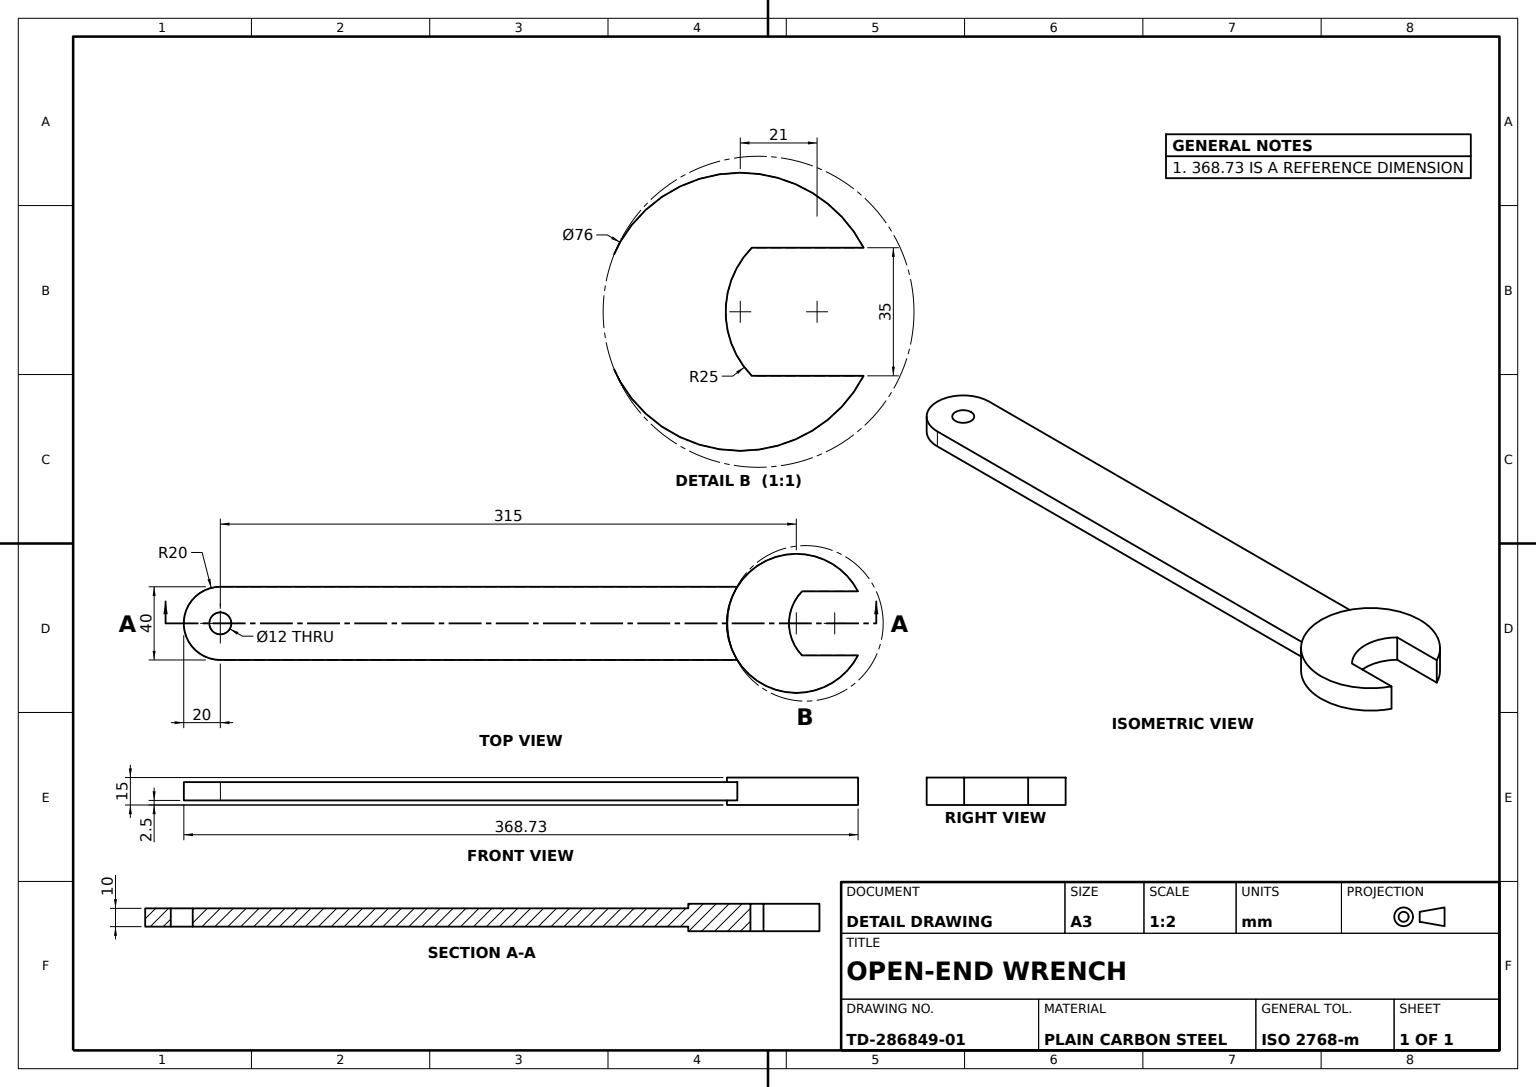
from build123d import *

# Parameters (mm, degrees)
WRENCH_OUTLINE_SKETCH_R  = 6
WRENCH_HANDLE_10MM_DEPTH = 5
JAW_HEAD_BOSS_15MM_DEPTH = 7.5


with BuildPart() as part:
    # Wrench Outline Sketch → Wrench Handle 10mm (new, symmetric)
    with BuildSketch(Plane(origin=(0, 0, 0), x_dir=(1, 0, 0), z_dir=(0, 1, 0))):
        with BuildLine():
            Line((125.189011157, 20), (-157.5, 20))
            ThreePointArc((-157.5, 20), (-177.5, 0), (-157.5, -20))
            Line((-157.5, -20), (125.189011157, -20))
            ThreePointArc((125.189011157, -20), (119.5, 0), (125.189011157, 20))
        make_face()
        with Locations(Location((-157.5, 0, 0), (0, 0, 270))):
            Circle(WRENCH_OUTLINE_SKETCH_R, mode=Mode.SUBTRACT)
    extrude(amount=WRENCH_HANDLE_10MM_DEPTH, both=True)

    # Jaw Head Sketch → Jaw Head Boss 15mm (add, symmetric)
    with BuildSketch(Plane(origin=(0, 0, 0), x_dir=(1, 0, 0), z_dir=(0, 1, 0))):
        with BuildLine():
            Line((160.646428929, -17.5), (191.230549951, -17.5))
            ThreePointArc((191.230549951, -17.5), (119.5, 0), (191.230549951, 17.5))
            Line((191.230549951, 17.5), (160.646428929, 17.5))
            ThreePointArc((160.646428929, 17.5), (153.5, 0), (160.646428929, -17.5))
        make_face()
    extrude(amount=JAW_HEAD_BOSS_15MM_DEPTH, both=True)


solid = part.part
